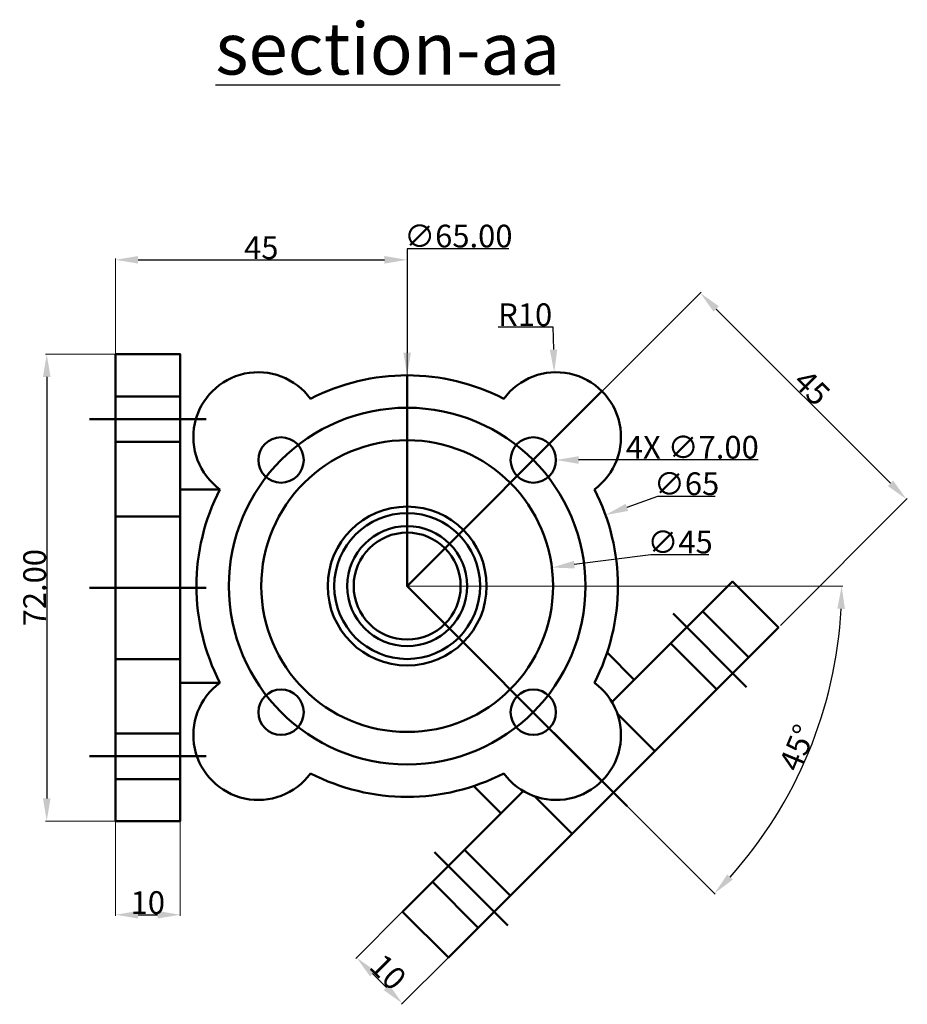
# Model space of a CAD drawing. Units: millimetres. Extents: x 75 to 489, y 21 to 350.
# Tile 1 of 5: x 133 to 270, y 21 to 173. Entities that reach past the tile are written whole.
import ezdxf

# ---------------------------------------------------------------- set-up
doc = ezdxf.new("R2010")
doc.units = ezdxf.units.MM
doc.header["$MEASUREMENT"] = 0
for name, color, linetype, lineweight in [('M-CONS', 9, 'Continuous', 13), ('M-DIMS', 2, 'Continuous', 25), ('M-OUTL', 7, 'Continuous', 50), ('M-TEXT', 7, 'Continuous', 25)]:
    doc.layers.add(name, color=color, linetype=linetype, lineweight=lineweight)
doc.styles.get("Standard").update_dxf_attribs({"font": 'arial.ttf'})
doc.dimstyles.get("Standard").update_dxf_attribs({"dimtxt": 3.5, "dimasz": 3.5, "dimexe": 0.18, "dimexo": 0.0625, "dimgap": 0.09, "dimtad": 1, "dimtoh": 1, "dimdec": 0, "dimzin": 0, "dimdsep": 46, "dimtxsty": 'Standard', "dimcen": 0.09, "dimclrd": 2, "dimclre": 251, "dimadec": 0, "dimazin": 0, "dimtfac": 1, "dimtdec": 0, "dimtofl": 0, "dimtmove": 0, "dimatfit": 3, "dimfxl": 1, "dimtolj": 1, "dimtzin": 0, "dimlwe": 5, "dimarcsym": 0})

# ---------------------------------------------------------------- blocks, each defined once
blk = doc.blocks.new('A$C3d481df2')
for p, q in [((14, 65.5), (4, 65.5)), ((18, 62), (0, 62)), ((14, 58.5), (4, 58.5)), ((14, 47), (4, 47)), ((18, 36), (0, 36)), ((14, 25), (4, 25)), ((14, 13.5), (4, 13.5)), ((18, 10), (0, 10)), ((14, 6.5), (4, 6.5))]:
    blk.add_line(p, q)
blk.add_lwpolyline([(4, 72), (4, 0), (14, 0), (14, 72)], close=True)
blk = doc.blocks.new('A$C01436580')
for p, q in [((13, 65.5), (3, 65.5)), ((16, 62), (0, 62)), ((13, 58.5), (3, 58.5)), ((13, 45), (4.86, 45)), ((16, 36), (0, 36)), ((13, 27), (4.86, 27)), ((13, 13.5), (3, 13.5)), ((16, 10), (0, 10)), ((13, 6.5), (3, 6.5))]:
    blk.add_line(p, q)
blk.add_lwpolyline([(3, 26.32), (3, 0), (13, 0), (13, 72), (3, 72), (3, 45.68)])
blk = doc.blocks.new('A$C8055e2f9')
at = {"ltscale": 5}
for q in [(49, 91.9), (79.05, 89.45), (79.05, 29.34)]:
    blk.add_line((49, 59.4), q, dxfattribs=at)
for p, q in [((20.12, 74.3), (14, 74.3)), ((79.84, 49.14), (84.04, 44.94)), ((20.12, 44.49), (14, 44.49)), ((59.26, 28.56), (63.46, 24.36))]:
    blk.add_line(p, q)
blk.add_circle((49, 59.4), 27.5, dxfattribs=at)
for centre, radius in [((29.55, 78.84), 3.5), ((68.45, 78.84), 3.5), ((49, 59.4), 22.5), ((49, 59.4), 12.25), ((49, 59.4), 11.25), ((49, 59.4), 9.25), ((49, 59.4), 8.25), ((29.55, 39.95), 3.5), ((68.45, 39.95), 3.5)]:
    blk.add_circle(centre, radius)
for centre, radius, start, end in [((26.02, 82.38), 10, 36.1501, 233.8499), ((49, 59.4), 32.5, 62.6998, 117.3002), ((71.98, 82.38), 10, 306.1501, 143.8499), ((49, 59.4), 32.5, 152.6998, 207.3002), ((49, 59.4), 32.5, 332.6998, 27.3002), ((26.02, 36.42), 10, 126.1501, 323.8499), ((71.98, 36.42), 10, 216.1501, 53.8499), ((49, 59.4), 32.5, 242.6998, 297.3002)]:
    blk.add_arc(centre, radius, start, end)
blk.add_blockref('A$C3d481df2', (0, 23.15))
at = {"rotation": 315.0000000000008}
blk.add_blockref('A$C01436580', (46.17, 11.31), dxfattribs=at)
blk = doc.blocks.new('*D36')
at = {"layer": 'Defpoints', "color": 0, "transparency": 16777216}
for p in [(192.4, 135.5), (147.4, 120.94), (192.4, 117.68)]:
    blk.add_point(p, dxfattribs=at)
at = {"layer": 'M-DIMS', "color": 0, "lineweight": 5, "transparency": 16777216}
for p, q in [((147.4, 121), (147.4, 135.68)), ((192.4, 117.74), (192.4, 135.68))]:
    blk.add_line(p, q, dxfattribs=at)
at = {"layer": 'M-DIMS', "color": 0, "lineweight": -2, "transparency": 16777216}
blk.add_line((150.9, 135.5), (188.9, 135.5), dxfattribs=at)
at = {"layer": 'M-DIMS', "color": 0, "transparency": 16777216}
for points in [[(150.9, 136.08), (150.9, 134.92), (147.4, 135.5)], [(188.9, 136.08), (188.9, 134.92), (192.4, 135.5)]]:
    blk.add_solid(points, dxfattribs=at)
at = {"layer": 'M-DIMS', "color": 0, "transparency": 16777216, "insert": (169.9, 137.37), "char_height": 3.5, "attachment_point": 5}
blk.add_mtext('\\A1;45', dxfattribs=at)
blk = doc.blocks.new('*D37')
at = {"layer": 'Defpoints', "color": 0, "transparency": 16777216}
for p in [(218.11, 110.89), (269.43, 98.57), (249.93, 79.07)]:
    blk.add_point(p, dxfattribs=at)
at = {"layer": 'M-DIMS', "color": 0, "lineweight": 5, "transparency": 16777216}
for p, q in [((218.16, 110.93), (237.74, 130.52)), ((249.98, 79.11), (269.56, 98.7))]:
    blk.add_line(p, q, dxfattribs=at)
at = {"layer": 'M-DIMS', "color": 0, "lineweight": -2, "transparency": 16777216}
blk.add_line((240.09, 127.91), (266.96, 101.04), dxfattribs=at)
at = {"layer": 'M-DIMS', "color": 0, "transparency": 16777216}
for points in [[(240.5, 128.33), (239.67, 127.5), (237.61, 130.39)], [(267.37, 101.46), (266.54, 100.63), (269.43, 98.57)]]:
    blk.add_solid(points, dxfattribs=at)
at = {"layer": 'M-DIMS', "color": 0, "transparency": 16777216, "insert": (254.84, 115.8), "char_height": 3.5, "attachment_point": 5, "rotation": 315}
blk.add_mtext('\\A1;45', dxfattribs=at)
blk = doc.blocks.new('*D38')
at = {"layer": 'Defpoints', "color": 0, "transparency": 16777216}
for p in [(192.4, 85.18), (192.4, 85.18), (231, 85.18), (222.46, 55.13), (250.45, 51.67)]:
    blk.add_point(p, dxfattribs=at)
at = {"layer": 'M-DIMS', "color": 0, "lineweight": 5, "transparency": 16777216}
for p, q in [((231.06, 85.18), (259.61, 85.18)), ((222.5, 55.09), (239.93, 37.66))]:
    blk.add_line(p, q, dxfattribs=at)
at = {"layer": 'M-DIMS', "color": 0, "lineweight": -2, "transparency": 16777216}
blk.add_arc((192.4, 85.18), 67.03, 317.9921, 357.0079, dxfattribs=at)
at = {"layer": 'M-DIMS', "color": 0, "transparency": 16777216}
for points in [[(258.76, 81.7), (259.93, 81.67), (259.43, 85.18)], [(242.63, 39.92), (241.79, 40.72), (239.8, 37.78)]]:
    blk.add_solid(points, dxfattribs=at)
at = {"layer": 'M-DIMS', "color": 0, "transparency": 16777216, "insert": (252.6, 60.25), "char_height": 3.5, "attachment_point": 5, "rotation": 67.5}
blk.add_mtext('\\A1;45°', dxfattribs=at)
blk = doc.blocks.new('*D39')
at = {"layer": 'Defpoints', "color": 0, "transparency": 16777216}
for p in [(191.7, 34.98), (198.77, 27.91), (191.68, 20.82)]:
    blk.add_point(p, dxfattribs=at)
at = {"layer": 'M-DIMS', "color": 0, "lineweight": 5, "transparency": 16777216}
for p, q in [((191.65, 34.93), (184.48, 27.76)), ((198.72, 27.86), (191.55, 20.69))]:
    blk.add_line(p, q, dxfattribs=at)
at = {"layer": 'M-DIMS', "color": 0, "lineweight": -2, "transparency": 16777216}
blk.add_line((187.08, 25.42), (189.21, 23.29), dxfattribs=at)
at = {"layer": 'M-DIMS', "color": 0, "transparency": 16777216}
for points in [[(187.5, 25.83), (186.67, 25), (184.61, 27.89)], [(189.62, 23.71), (188.79, 22.88), (191.68, 20.82)]]:
    blk.add_solid(points, dxfattribs=at)
at = {"layer": 'M-DIMS', "color": 0, "transparency": 16777216, "insert": (189.47, 25.68), "char_height": 3.5, "attachment_point": 5, "rotation": 315}
blk.add_mtext('\\A1;10', dxfattribs=at)
blk = doc.blocks.new('*D40')
at = {"layer": 'Defpoints', "color": 0, "transparency": 16777216}
for p in [(147.4, 48.94), (157.4, 48.94), (157.4, 34.5)]:
    blk.add_point(p, dxfattribs=at)
at = {"layer": 'M-DIMS', "color": 0, "lineweight": 5, "transparency": 16777216}
for p, q in [((147.4, 48.88), (147.4, 34.32)), ((157.4, 48.88), (157.4, 34.32))]:
    blk.add_line(p, q, dxfattribs=at)
at = {"layer": 'M-DIMS', "color": 0, "lineweight": -2, "transparency": 16777216}
blk.add_line((150.9, 34.5), (153.9, 34.5), dxfattribs=at)
at = {"layer": 'M-DIMS', "color": 0, "transparency": 16777216}
for points in [[(150.9, 35.08), (150.9, 33.92), (147.4, 34.5)], [(153.9, 35.08), (153.9, 33.92), (157.4, 34.5)]]:
    blk.add_solid(points, dxfattribs=at)
at = {"layer": 'M-DIMS', "color": 0, "transparency": 16777216, "insert": (152.4, 36.38), "char_height": 3.5, "attachment_point": 5}
blk.add_mtext('\\A1;10', dxfattribs=at)
blk = doc.blocks.new('*D41')
at = {"layer": 'Defpoints', "color": 0, "transparency": 16777216}
for p in [(223, 96.14), (161.81, 74.23)]:
    blk.add_point(p, dxfattribs=at)
at = {"layer": 'M-DIMS', "color": 0, "lineweight": -2, "transparency": 16777216}
for p, q in [((231, 99), (226.3, 97.32)), ((239.94, 99), (231, 99))]:
    blk.add_line(p, q, dxfattribs=at)
at = {"layer": 'M-DIMS', "color": 0, "lineweight": 5, "transparency": 16777216}
for p, q in [((192.31, 85.18), (192.49, 85.18)), ((192.4, 85.09), (192.4, 85.27))]:
    blk.add_line(p, q, dxfattribs=at)
at = {"layer": 'M-DIMS', "color": 0, "transparency": 16777216}
blk.add_solid([(226.1, 97.87), (226.49, 96.77), (223, 96.14)], dxfattribs=at)
at = {"layer": 'M-DIMS', "color": 0, "transparency": 16777216, "insert": (235.51, 100.97), "char_height": 3.5, "attachment_point": 5}
blk.add_mtext('\\A1;∅65', dxfattribs=at)
blk = doc.blocks.new('*D42')
at = {"layer": 'Defpoints', "color": 0, "transparency": 16777216}
for p in [(214.72, 88.04), (170.09, 82.32)]:
    blk.add_point(p, dxfattribs=at)
at = {"layer": 'M-DIMS', "color": 0, "lineweight": -2, "transparency": 16777216}
for p, q in [((230, 90), (218.19, 88.49)), ((238.94, 90), (230, 90))]:
    blk.add_line(p, q, dxfattribs=at)
at = {"layer": 'M-DIMS', "color": 0, "lineweight": 5, "transparency": 16777216}
for p, q in [((192.31, 85.18), (192.49, 85.18)), ((192.4, 85.09), (192.4, 85.27))]:
    blk.add_line(p, q, dxfattribs=at)
at = {"layer": 'M-DIMS', "color": 0, "transparency": 16777216}
blk.add_solid([(218.12, 89.07), (218.27, 87.91), (214.72, 88.04)], dxfattribs=at)
at = {"layer": 'M-DIMS', "color": 0, "transparency": 16777216, "insert": (234.51, 91.97), "char_height": 3.5, "attachment_point": 5}
blk.add_mtext('\\A1;∅45', dxfattribs=at)
blk = doc.blocks.new('*D43')
at = {"layer": 'Defpoints', "color": 0, "transparency": 16777216}
for p in [(215.09, 118.16), (215.38, 108.16)]:
    blk.add_point(p, dxfattribs=at)
at = {"layer": 'M-DIMS', "color": 0, "lineweight": -2, "transparency": 16777216}
for p, q in [((206.43, 125.16), (214.88, 125.16)), ((214.88, 125.16), (214.98, 121.66))]:
    blk.add_line(p, q, dxfattribs=at)
at = {"layer": 'M-DIMS', "color": 0, "lineweight": 5, "transparency": 16777216}
for p, q in [((215.29, 108.16), (215.47, 108.16)), ((215.38, 108.07), (215.38, 108.25))]:
    blk.add_line(p, q, dxfattribs=at)
at = {"layer": 'M-DIMS', "color": 0, "transparency": 16777216}
blk.add_solid([(215.56, 121.67), (214.4, 121.64), (215.09, 118.16)], dxfattribs=at)
at = {"layer": 'M-DIMS', "color": 0, "transparency": 16777216, "insert": (210.61, 127.03), "char_height": 3.5, "attachment_point": 5}
blk.add_mtext('\\A1;R10', dxfattribs=at)
blk = doc.blocks.new('*D64')
at = {"layer": 'Defpoints', "color": 0, "transparency": 16777216}
for p in [(147.4, 120.94), (136.8, 48.94), (147.4, 48.94)]:
    blk.add_point(p, dxfattribs=at)
at = {"layer": 'M-DIMS', "color": 251, "lineweight": 5, "transparency": 16777216}
for p, q in [((147.34, 120.94), (136.62, 120.94)), ((147.34, 48.94), (136.62, 48.94))]:
    blk.add_line(p, q, dxfattribs=at)
at = {"layer": 'M-DIMS', "color": 2, "lineweight": -2, "transparency": 16777216}
blk.add_line((136.8, 117.44), (136.8, 52.44), dxfattribs=at)
at = {"layer": 'M-DIMS', "color": 2, "transparency": 16777216}
for points in [[(136.22, 117.44), (137.39, 117.44), (136.8, 120.94)], [(136.22, 52.44), (137.39, 52.44), (136.8, 48.94)]]:
    blk.add_solid(points, dxfattribs=at)
at = {"layer": 'M-DIMS', "color": 0, "transparency": 16777216, "insert": (134.93, 84.94), "char_height": 3.5, "attachment_point": 5, "rotation": 90}
blk.add_mtext('\\A1;72.00', dxfattribs=at)
blk = doc.blocks.new('*D70')
at = {"layer": 'Defpoints', "color": 0, "transparency": 16777216}
for p in [(192.4, 117.68), (192.4, 52.68)]:
    blk.add_point(p, dxfattribs=at)
at = {"layer": 'M-DIMS', "color": 2, "lineweight": -2, "transparency": 16777216}
for p, q in [((208.1, 137.18), (192.4, 137.18)), ((192.4, 137.18), (192.4, 121.18))]:
    blk.add_line(p, q, dxfattribs=at)
at = {"layer": 'M-DIMS', "color": 251, "lineweight": 5, "transparency": 16777216}
for p, q in [((192.31, 85.18), (192.49, 85.18)), ((192.4, 85.09), (192.4, 85.27))]:
    blk.add_line(p, q, dxfattribs=at)
at = {"layer": 'M-DIMS', "color": 2, "transparency": 16777216}
blk.add_solid([(191.82, 121.18), (192.99, 121.18), (192.4, 117.68)], dxfattribs=at)
at = {"layer": 'M-DIMS', "color": 0, "transparency": 16777216, "insert": (200.3, 139.16), "char_height": 3.5, "attachment_point": 5}
blk.add_mtext('\\A1;∅65.00', dxfattribs=at)
blk = doc.blocks.new('*D71')
at = {"layer": 'Defpoints', "color": 0, "transparency": 16777216}
for p in [(208.35, 104.63), (215.35, 104.63)]:
    blk.add_point(p, dxfattribs=at)
at = {"layer": 'M-DIMS', "color": 251, "lineweight": 5, "transparency": 16777216}
for p, q in [((211.76, 104.63), (211.94, 104.63)), ((211.85, 104.54), (211.85, 104.72))]:
    blk.add_line(p, q, dxfattribs=at)
at = {"layer": 'M-DIMS', "color": 2, "lineweight": -2, "transparency": 16777216}
for p, q in [((226.12, 104.63), (218.85, 104.63)), ((246.57, 104.63), (226.12, 104.63))]:
    blk.add_line(p, q, dxfattribs=at)
at = {"layer": 'M-DIMS', "color": 2, "transparency": 16777216}
blk.add_solid([(218.85, 105.21), (218.85, 104.04), (215.35, 104.63)], dxfattribs=at)
at = {"layer": 'M-DIMS', "color": 0, "transparency": 16777216, "insert": (236.39, 106.6), "char_height": 3.5, "attachment_point": 5}
blk.add_mtext('\\A1;4X ∅7.00', dxfattribs=at)

msp = doc.modelspace()

# ---------------------------------------------------------------- linework, layer by layer
at = {"layer": 'M-CONS'}
msp.add_line((192.404, 85.182), (231, 85.182), dxfattribs=at)

# ---------------------------------------------------------------- block references
at = {"layer": 'M-OUTL'}
msp.add_blockref('A$C8055e2f9', (143.404, 25.785), dxfattribs=at)

# ---------------------------------------------------------------- texts
at = {"layer": 'M-TEXT', "insert": (162.816, 172.069), "char_height": 8, "attachment_point": 1}
msp.add_mtext_dynamic_manual_height_columns('{\\Lsection-aa}', width=43.19704, gutter_width=1, heights=[0], dxfattribs=at)

# ---------------------------------------------------------------- dimensions: what is measured, and where the dimension line sits
at = {"layer": 'M-DIMS'}
for p1, p2, override, picture, middle in [((192.404, 52.682), (192.404, 117.682), {"dimdec": 2, "dimlfac": 1, "dimrnd": 0, "dimzin": 0, "dimdsep": 46, "dimlunit": 2}, '*D70', (200.297, 137.182)), ((161.806, 74.227), (223.002, 96.137), {"dimclrd": 0, "dimclre": 0, "dimclrt": 0}, '*D41', (235.514, 99)), ((170.086, 82.322), (214.721, 88.042), {"dimclrd": 0, "dimclre": 0, "dimclrt": 0}, '*D42', (230, 90))]:
    dim = msp.add_diameter_dim_2p(p1=p1, p2=p2, dimstyle='Standard', override=override, dxfattribs=at)
    dim.commit()
    dim.dimension.update_dxf_attribs({"geometry": picture, "text_midpoint": middle, "dimtype": 163})
for base, p1, p2, picture, middle in [((192.404, 135.5), (147.404, 120.938), (192.404, 117.682), '*D36', (169.904, 137.37)), ((157.404, 34.5), (147.404, 48.938), (157.404, 48.938), '*D40', (152.404, 36.377))]:
    dim = msp.add_linear_dim(base=base, p1=p1, p2=p2, dimstyle='Standard', override={"dimclrd": 0, "dimclre": 0, "dimclrt": 0}, dxfattribs=at)
    dim.commit()
    dim.dimension.update_dxf_attribs({"geometry": picture, "text_midpoint": middle})
dim = msp.add_radius_dim(center=(215.385, 108.163), mpoint=(215.085, 118.158), dimstyle='Standard', override={"dimclrd": 0, "dimclre": 0, "dimclrt": 0}, dxfattribs=at)
dim.commit()
dim.dimension.update_dxf_attribs({"geometry": '*D43', "text_midpoint": (210.61, 127.032)})
for p1, p2, distance, picture, middle in [((218.111, 110.889), (249.931, 79.069), 27.577, '*D37', (254.843, 115.801)), ((191.697, 34.977), (198.768, 27.906), -10.022, '*D39', (189.473, 25.682))]:
    dim = msp.add_aligned_dim(p1=p1, p2=p2, distance=distance, dimstyle='Standard', override={"dimclrd": 0, "dimclre": 0, "dimclrt": 0}, dxfattribs=at)
    dim.commit()
    dim.dimension.update_dxf_attribs({"geometry": picture, "text_midpoint": middle})
dim = msp.add_linear_dim(base=(136.804, 48.938), p1=(147.404, 120.938), p2=(147.404, 48.938), angle=90, dimstyle='Standard', override={"dimdec": 2, "dimlfac": 1, "dimrnd": 0, "dimzin": 0, "dimdsep": 46, "dimlunit": 2}, dxfattribs=at)
dim.commit()
dim.dimension.update_dxf_attribs({"geometry": '*D64', "text_midpoint": (134.927, 84.938)})
dim = msp.add_diameter_dim_2p(p1=(208.349, 104.627), p2=(215.349, 104.627), text='4X <>', dimstyle='Standard', override={"dimdec": 2, "dimlfac": 1, "dimrnd": 0, "dimzin": 0, "dimdsep": 46, "dimlunit": 2}, dxfattribs=at)
dim.commit()
dim.dimension.update_dxf_attribs({"geometry": '*D71', "text_midpoint": (226.119, 104.627), "dimtype": 163})
dim = msp.add_angular_dim_2l(base=(250.454, 51.667), line1=((192.404, 85.182), (222.456, 55.13)), line2=((192.404, 85.182), (231, 85.182)), dimstyle='Standard', override={"dimclrd": 0, "dimclre": 0, "dimclrt": 0}, dxfattribs=at)
dim.commit()
dim.dimension.update_dxf_attribs({"geometry": '*D38', "text_midpoint": (252.604, 60.246)})

doc.saveas('drawing.dxf')
